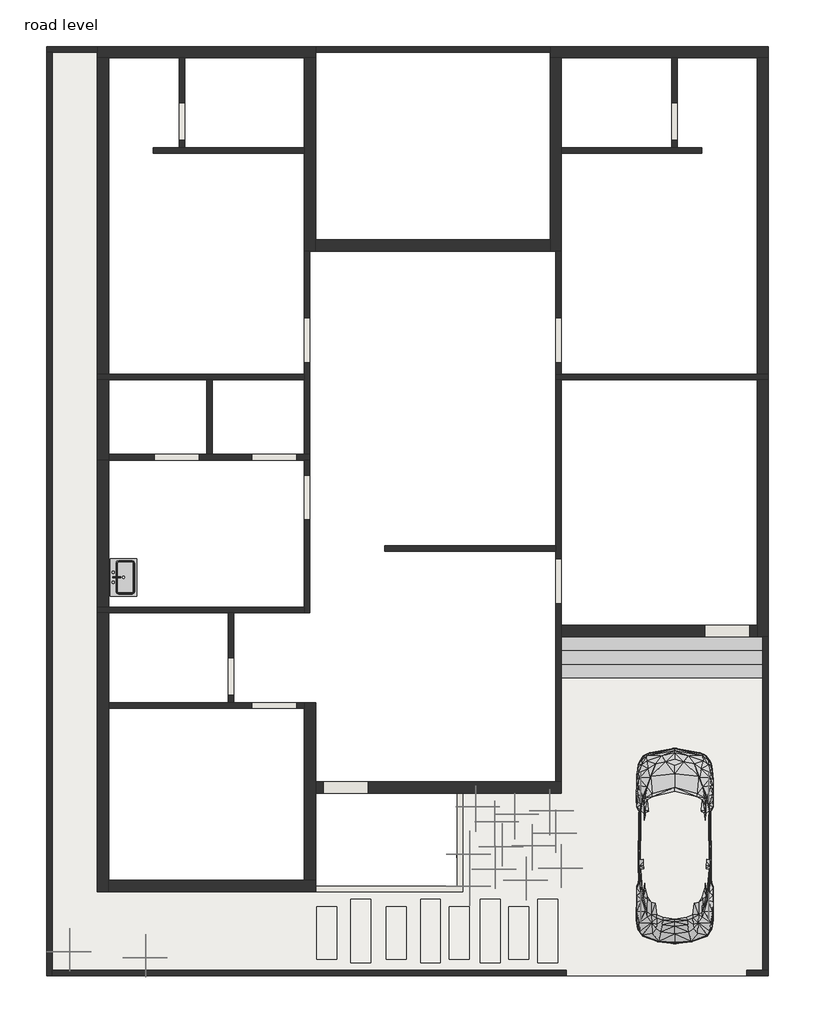
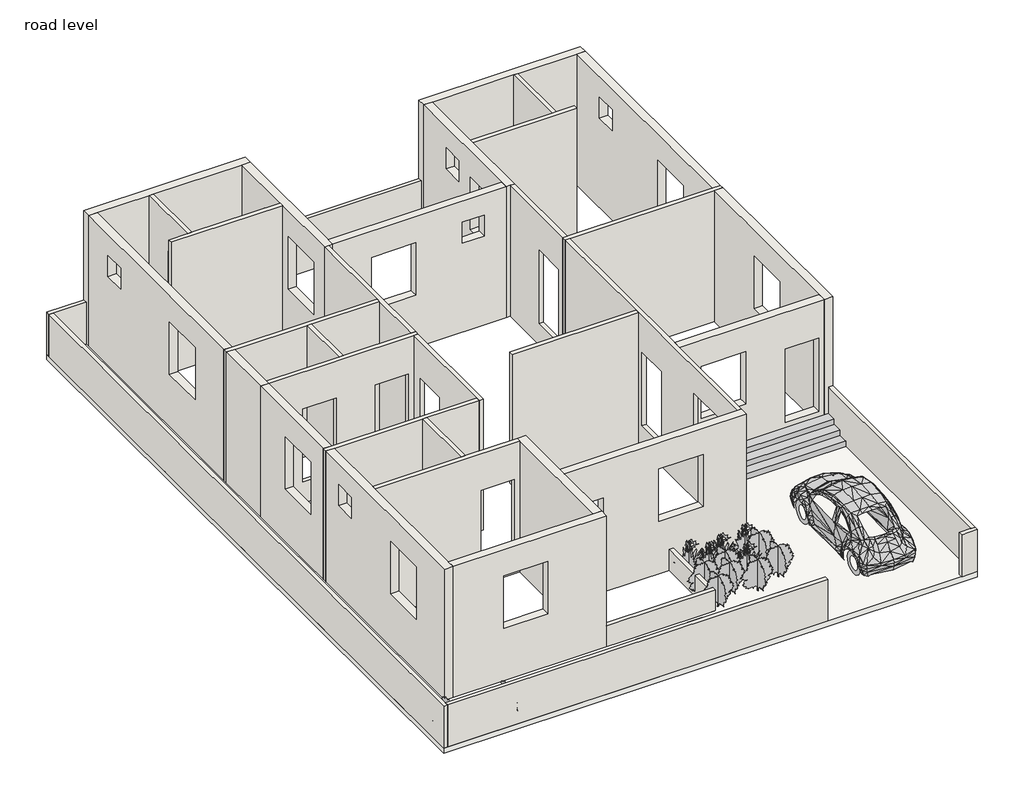
# One storey: 39 walls, 14 geographic elements, 2 slabs, 1 flow terminal, 1 furniture element, 1 proxy.
# Revit data of these elements (continued)
# Type (continued)
#   Layers, outside or top first: 0' - 4" "Asphalt Shingle" (function 1)
# Type
#   Assembly Code = "B1010"
#   Function = 0
#   Layers, outside or top first: 0' - 6" "Concrete, Cast-in-Place gray" (function 1)
# Type
#   Assembly Code = "B2010"
#   Layers, outside or top first: 0' - 9" no material (function 1)
# Type
#   Assembly Code = "B2010"
#   Layers, outside or top first: 0' - 4 1/2" no material (function 1)
# Element 1 (IfcBuildingElementProxy, "RPC Beetle : RPC Beetle")
#   Phase Created = New Construction
# Element 2 (IfcFlowTerminal, "Sink Kitchen-Single : 30\" x 21\"")
#   Mark = "7"
#   Phase Created = New Construction
#   Materials on its faces: "Steel, Polished"
# Element 3 (IfcFurniture, "Casework 15 : Casework 15")
#   Phase Created = New Construction
# Elements 4, 5, 6, 7, 8 (IfcGeographicElement, "RPC Plant - Tropical")
#   Phase Created = New Construction
# Elements 9, 10, 11, 12, 13, 14, 15, 16, 17 (IfcGeographicElement, "RPC Plant - Tropical : Jungle Flame - 3'")
#   Phase Created = New Construction
# Element 18 (IfcSlab)
#   Height Offset From Level = 0' - 2"
#   Phase Created = New Construction
#   Materials on its faces: "Asphalt Shingle"
# Element 19 (IfcSlab)
#   Height Offset From Level = 0' - 0"
#   Phase Created = New Construction
#   Materials on its faces: "Concrete, Cast-in-Place gray"
# Elements 20, 21, 22, 23, 24, 25, 26, 27, 28, 29, 30, 31, 32, 33, 34, 35, 36, 37, 38, 39, 40, 41, 42, 43, 44, 45, 46, 47, 53, 54, 55 (IfcWall)
#   Top Offset = 0' - 0"
#   Base Offset = 0' - 0"
#   wall height = 12' - 6"
#   Phase Created = New Construction
#   Base Constraint = road level
#   Top Constraint = terrace
#   Materials on its faces: "Default Wall"
# Elements 48, 49, 50, 51, 58 (IfcWall)
#   Top Offset = 0' - 0"
#   Base Offset = 0' - 0"
#   Unconnected Height = 4' - 0"
#   wall height = 4' - 0"
#   Phase Created = New Construction
#   Base Constraint = road level
#   Materials on its faces: "Default Wall"
# Element 52 (IfcWall)
#   Top Offset = 0' - 0"
#   Base Offset = 0' - 0"
#   Unconnected Height = 5' - 0"
#   wall height = 5' - 0"
#   Phase Created = New Construction
#   Base Constraint = road level
#   Materials on its faces: "Default Wall"
# Elements 56, 57 (IfcWall)
#   Top Offset = 0' - 0"
#   Base Offset = 0' - 0"
#   wall height = 2' - 0"
#   Phase Created = New Construction
#   Base Constraint = road level
#   Top Constraint = ground floor or plinth
#   Materials on its faces: "Default Wall"
# Materials
#   "Steel, Polished": class "Metal", colour RGB 57 57 57, transparency 0, Description = "Polished steel", Cost = 0
#   "Asphalt Shingle": class "Generic", colour RGB 155 155 155, transparency 0, Description = "Asphalt roofing shingle", Cost = 0
#   "Concrete, Cast-in-Place gray": class "Concrete", colour RGB 192 192 192, transparency 0, Description = "Cast-in-place concrete", Cost = 0
#   "Default Wall": colour RGB 128 128 128, transparency 0, Cost = 0
